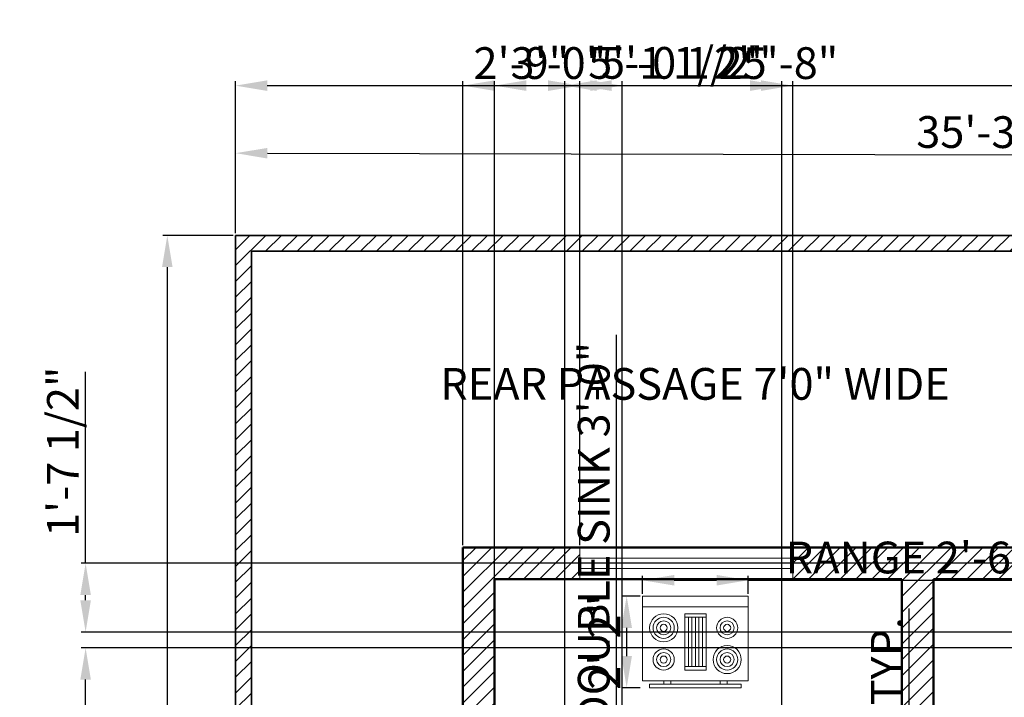
# Model space of a CAD drawing. Units: inches. Extents: x 36184 to 36805, y 18177 to 19069.
# Tile 4 of 5: x 36184 to 36463, y 18876 to 19069. Entities that reach past the tile are written whole.
import ezdxf

# ---------------------------------------------------------------- set-up
doc = ezdxf.new("R2010")
doc.units = ezdxf.units.IN
for name, color, linetype, lineweight in [('A-ANNO-DIMS', 2, 'Continuous', 18), ('A-AREA-IDEN', 7, 'Continuous', 25), ('A-EQPM', 8, 'Continuous', 18), ('A-GLAZ', 4, 'Continuous', 18), ('A-WALL', 7, 'Continuous', 50), ('C-PROP', 7, 'Continuous', 35), ('L-SITE-WALL', 7, 'Continuous', 35)]:
    doc.layers.add(name, color=color, linetype=linetype, lineweight=lineweight)
doc.layers.add('A-WALL-PATT', color=244, linetype='Continuous', lineweight=13, true_color=0x991b1e)
doc.styles.get("Standard").update_dxf_attribs({"font": 'arial.ttf'})
doc.dimstyles.new('ISO-25', dxfattribs={"dimtxt": 9, "dimasz": 9, "dimexe": 1.25, "dimexo": 0.625, "dimtad": 1, "dimdec": 1, "dimrnd": 9, "dimlunit": 3, "dimtxsty": 'Standard', "dimcen": 2.5, "dimadec": 0, "dimazin": 0, "dimtfac": 1, "dimtdec": 1, "dimtmove": 0, "dimatfit": 3, "dimfxl": 1, "dimarcsym": 0})

# ---------------------------------------------------------------- blocks, each defined once
blk = doc.blocks.new('Range-Oven - 30 in top')
for p, q in [((0, -3), (30, -3)), ((12, -6), (18, -6)), ((13, -20), (13, -6)), ((14, -6), (14, -20)), ((15, -20), (15, -6)), ((16, -6), (16, -20)), ((17, -20), (17, -6)), ((18, -20), (12, -20)), ((6, -24), (6, -25)), ((8, -25), (8, -24)), ((22, -25), (22, -24)), ((24, -24), (24, -25))]:
    blk.add_line(p, q)
for points in [[(0, -24), (0, 0), (30, 0), (30, -24)], [(12, -21), (12, -5), (18, -5), (18, -21)], [(2, -26), (2, -25), (28, -25), (28, -26)]]:
    blk.add_lwpolyline(points, close=True)
for centre, radius in [((6, -9), 4), ((6, -9), 3), ((6, -9), 2), ((6, -9), 1), ((24, -9), 3), ((24, -9), 2), ((24, -9), 1), ((6, -18), 3), ((6, -18), 2), ((24, -18), 4), ((24, -18), 3), ((24, -18), 2), ((6, -18), 1), ((24, -18), 1)]:
    blk.add_circle(centre, radius)
blk = doc.blocks.new('*D13')
at = {"layer": 'A-ANNO-DIMS', "color": 0, "lineweight": -2, "transparency": 16777216}
for p, q in [((36245.31, 19007.93), (36245.36, 19031.89)), ((36665.31, 19007.11), (36665.36, 19031.07)), ((36254.36, 19030.62), (36656.36, 19029.84))]:
    blk.add_line(p, q, dxfattribs=at)
at = {"layer": 'A-ANNO-DIMS', "color": 0, "transparency": 16777216}
for points in [[(36254.36, 19032.12), (36254.35, 19029.12), (36245.36, 19030.64)], [(36656.36, 19031.34), (36656.35, 19028.34), (36665.36, 19029.82)]]:
    blk.add_solid(points, dxfattribs=at)
at = {"layer": 'Defpoints', "color": 0, "transparency": 16777216}
for p in [(36665.36, 19029.82), (36245.31, 19007.3), (36665.31, 19006.48)]:
    blk.add_point(p, dxfattribs=at)
at = {"layer": 'A-ANNO-DIMS', "color": 0, "transparency": 16777216, "insert": (36455.37, 19035.45), "char_height": 9, "attachment_point": 5, "rotation": 359.8885}
blk.add_mtext('35\'-3"', dxfattribs=at)
blk = doc.blocks.new('*D14')
at = {"layer": 'A-ANNO-DIMS', "color": 0, "lineweight": -2, "transparency": 16777216}
for p, q in [((36244.69, 19007.3), (36224.73, 19007.3)), ((36225.98, 18998.3), (36225.98, 18420.79)), ((36244.69, 18411.79), (36224.73, 18411.79))]:
    blk.add_line(p, q, dxfattribs=at)
at = {"layer": 'A-ANNO-DIMS', "color": 0, "transparency": 16777216}
for points in [[(36224.48, 18998.3), (36227.48, 18998.3), (36225.98, 19007.3)], [(36224.48, 18420.79), (36227.48, 18420.79), (36225.98, 18411.79)]]:
    blk.add_solid(points, dxfattribs=at)
at = {"layer": 'Defpoints', "color": 0, "transparency": 16777216}
for p in [(36245.31, 19007.3), (36225.98, 18411.79), (36245.31, 18411.79)]:
    blk.add_point(p, dxfattribs=at)
at = {"layer": 'A-ANNO-DIMS', "color": 0, "transparency": 16777216, "insert": (36220.76, 18709.54), "char_height": 9, "attachment_point": 5, "rotation": 90}
blk.add_mtext('49\'-6"', dxfattribs=at)
blk = doc.blocks.new('*D28')
at = {"layer": 'A-ANNO-DIMS', "color": 0, "lineweight": -2, "transparency": 16777216}
for p, q in [((36436.4, 18801.8), (36436.4, 18901.45)), ((36431.63, 18801.8), (36437.65, 18801.8)), ((36436.4, 18774.8), (36436.4, 18792.8)), ((36431.63, 18765.8), (36437.65, 18765.8))]:
    blk.add_line(p, q, dxfattribs=at)
at = {"layer": 'A-ANNO-DIMS', "color": 0, "transparency": 16777216}
for points in [[(36434.9, 18792.8), (36437.9, 18792.8), (36436.4, 18801.8)], [(36434.9, 18774.8), (36437.9, 18774.8), (36436.4, 18765.8)]]:
    blk.add_solid(points, dxfattribs=at)
at = {"layer": 'Defpoints', "color": 0, "transparency": 16777216}
for p in [(36431, 18801.8), (36436.4, 18801.8), (36431, 18765.8)]:
    blk.add_point(p, dxfattribs=at)
at = {"layer": 'A-ANNO-DIMS', "color": 0, "transparency": 16777216, "insert": (36431.18, 18856.13), "char_height": 9, "attachment_point": 5, "rotation": 90}
blk.add_mtext('LEAF 3\'-0" TYP.', dxfattribs=at)
blk = doc.blocks.new('*D40')
at = {"layer": 'A-ANNO-DIMS', "color": 0, "lineweight": -2, "transparency": 16777216}
for p, q in [((36360.76, 18905.62), (36360.76, 18910.74)), ((36369.76, 18909.49), (36381.76, 18909.49)), ((36390.76, 18905.62), (36390.76, 18910.74)), ((36390.76, 18909.49), (36472.67, 18909.49))]:
    blk.add_line(p, q, dxfattribs=at)
at = {"layer": 'A-ANNO-DIMS', "color": 0, "transparency": 16777216}
for points in [[(36369.76, 18910.99), (36369.76, 18907.99), (36360.76, 18909.49)], [(36381.76, 18910.99), (36381.76, 18907.99), (36390.76, 18909.49)]]:
    blk.add_solid(points, dxfattribs=at)
at = {"layer": 'Defpoints', "color": 0, "transparency": 16777216}
for p in [(36390.76, 18909.49), (36360.76, 18904.99), (36390.76, 18904.99)]:
    blk.add_point(p, dxfattribs=at)
at = {"layer": 'A-ANNO-DIMS', "color": 0, "transparency": 16777216, "insert": (36436.22, 18914.77), "char_height": 9, "attachment_point": 5}
blk.add_mtext('RANGE 2\'-6"', dxfattribs=at)
blk = doc.blocks.new('*D41')
at = {"layer": 'A-ANNO-DIMS', "color": 0, "lineweight": -2, "transparency": 16777216}
for p, q in [((36360.13, 18904.99), (36355.01, 18904.99)), ((36356.26, 18887.99), (36356.26, 18895.99)), ((36360.13, 18878.99), (36355.01, 18878.99))]:
    blk.add_line(p, q, dxfattribs=at)
at = {"layer": 'A-ANNO-DIMS', "color": 0, "transparency": 16777216}
for points in [[(36354.76, 18895.99), (36357.76, 18895.99), (36356.26, 18904.99)], [(36354.76, 18887.99), (36357.76, 18887.99), (36356.26, 18878.99)]]:
    blk.add_solid(points, dxfattribs=at)
at = {"layer": 'Defpoints', "color": 0, "transparency": 16777216}
for p in [(36356.26, 18904.99), (36360.76, 18904.99), (36360.76, 18878.99)]:
    blk.add_point(p, dxfattribs=at)
at = {"layer": 'A-ANNO-DIMS', "color": 0, "transparency": 16777216, "insert": (36351.12, 18891.99), "char_height": 9, "attachment_point": 5, "rotation": 90}
blk.add_mtext('2\'-2"', dxfattribs=at)
blk = doc.blocks.new('*D42')
at = {"layer": 'A-ANNO-DIMS', "color": 0, "lineweight": -2, "transparency": 16777216}
for p, q in [((36353.36, 18857.38), (36353.36, 18979.14)), ((36348.59, 18857.38), (36354.61, 18857.38)), ((36353.36, 18830.38), (36353.36, 18848.38)), ((36348.59, 18821.38), (36354.61, 18821.38))]:
    blk.add_line(p, q, dxfattribs=at)
at = {"layer": 'A-ANNO-DIMS', "color": 0, "transparency": 16777216}
for points in [[(36351.86, 18848.38), (36354.86, 18848.38), (36353.36, 18857.38)], [(36351.86, 18830.38), (36354.86, 18830.38), (36353.36, 18821.38)]]:
    blk.add_solid(points, dxfattribs=at)
at = {"layer": 'Defpoints', "color": 0, "transparency": 16777216}
for p in [(36347.96, 18857.38), (36353.36, 18857.38), (36347.96, 18821.38)]:
    blk.add_point(p, dxfattribs=at)
at = {"layer": 'A-ANNO-DIMS', "color": 0, "transparency": 16777216, "insert": (36348.08, 18922.76), "char_height": 9, "attachment_point": 5, "rotation": 90}
blk.add_mtext('DOUBLE SINK 3\'-0"', dxfattribs=at)
blk = doc.blocks.new('*D45')
at = {"layer": 'A-ANNO-DIMS', "color": 0, "lineweight": -2, "transparency": 16777216}
for p, q in [((36245.31, 19007.93), (36245.31, 19051.05)), ((36553.31, 19007.93), (36553.31, 19051.05)), ((36254.31, 19049.8), (36544.31, 19049.8))]:
    blk.add_line(p, q, dxfattribs=at)
at = {"layer": 'A-ANNO-DIMS', "color": 0, "transparency": 16777216}
for points in [[(36254.31, 19051.3), (36254.31, 19048.3), (36245.31, 19049.8)], [(36544.31, 19051.3), (36544.31, 19048.3), (36553.31, 19049.8)]]:
    blk.add_solid(points, dxfattribs=at)
at = {"layer": 'Defpoints', "color": 0, "transparency": 16777216}
for p in [(36553.31, 19049.8), (36245.31, 19007.3), (36553.31, 19007.3)]:
    blk.add_point(p, dxfattribs=at)
at = {"layer": 'A-ANNO-DIMS', "color": 0, "transparency": 16777216, "insert": (36399.31, 19055.02), "char_height": 9, "attachment_point": 5}
blk.add_mtext('25\'-8"', dxfattribs=at)
blk = doc.blocks.new('*D49')
at = {"layer": 'A-ANNO-DIMS', "color": 0, "lineweight": -2, "transparency": 16777216}
for p, q in [((36600.19, 18890.3), (36201.56, 18890.3)), ((36202.81, 18839.3), (36202.81, 18881.3)), ((36600.19, 18830.3), (36201.56, 18830.3))]:
    blk.add_line(p, q, dxfattribs=at)
at = {"layer": 'A-ANNO-DIMS', "color": 0, "transparency": 16777216}
for points in [[(36201.31, 18881.3), (36204.31, 18881.3), (36202.81, 18890.3)], [(36201.31, 18839.3), (36204.31, 18839.3), (36202.81, 18830.3)]]:
    blk.add_solid(points, dxfattribs=at)
at = {"layer": 'Defpoints', "color": 0, "transparency": 16777216}
for p in [(36202.81, 18890.3), (36600.81, 18890.3), (36600.81, 18830.3)]:
    blk.add_point(p, dxfattribs=at)
at = {"layer": 'A-ANNO-DIMS', "color": 0, "transparency": 16777216, "insert": (36197.59, 18860.3), "char_height": 9, "attachment_point": 5, "rotation": 90}
blk.add_mtext('5\'-0"', dxfattribs=at)
blk = doc.blocks.new('*D50')
at = {"layer": 'A-ANNO-DIMS', "color": 0, "lineweight": -2, "transparency": 16777216}
for p, q in [((36202.81, 18914.3), (36202.81, 18968.6)), ((36600.19, 18914.3), (36201.56, 18914.3)), ((36202.81, 18903.8), (36202.81, 18905.3)), ((36600.19, 18894.8), (36201.56, 18894.8))]:
    blk.add_line(p, q, dxfattribs=at)
at = {"layer": 'A-ANNO-DIMS', "color": 0, "transparency": 16777216}
for points in [[(36201.31, 18905.3), (36204.31, 18905.3), (36202.81, 18914.3)], [(36201.31, 18903.8), (36204.31, 18903.8), (36202.81, 18894.8)]]:
    blk.add_solid(points, dxfattribs=at)
at = {"layer": 'Defpoints', "color": 0, "transparency": 16777216}
for p in [(36202.81, 18914.3), (36600.81, 18914.3), (36600.81, 18894.8)]:
    blk.add_point(p, dxfattribs=at)
at = {"layer": 'A-ANNO-DIMS', "color": 0, "transparency": 16777216, "insert": (36197.53, 18945.95), "char_height": 9, "attachment_point": 5, "rotation": 90}
blk.add_mtext('1\'-7 1/2"', dxfattribs=at)
blk = doc.blocks.new('*D53')
at = {"layer": 'A-ANNO-DIMS', "color": 0, "lineweight": -2, "transparency": 16777216}
for p, q in [((36342.97, 18919.43), (36342.97, 19051.05)), ((36403.35, 18919.43), (36403.35, 19051.05)), ((36351.97, 19049.8), (36394.35, 19049.8))]:
    blk.add_line(p, q, dxfattribs=at)
at = {"layer": 'A-ANNO-DIMS', "color": 0, "transparency": 16777216}
for points in [[(36351.97, 19051.3), (36351.97, 19048.3), (36342.97, 19049.8)], [(36394.35, 19051.3), (36394.35, 19048.3), (36403.35, 19049.8)]]:
    blk.add_solid(points, dxfattribs=at)
at = {"layer": 'Defpoints', "color": 0, "transparency": 16777216}
for p in [(36403.35, 19049.8), (36342.97, 18918.8), (36403.35, 18918.8)]:
    blk.add_point(p, dxfattribs=at)
at = {"layer": 'A-ANNO-DIMS', "color": 0, "transparency": 16777216, "insert": (36373.16, 19055.08), "char_height": 9, "attachment_point": 5}
blk.add_mtext('5\'-0 1/2"', dxfattribs=at)
blk = doc.blocks.new('*D54')
at = {"layer": 'A-ANNO-DIMS', "color": 0, "lineweight": -2, "transparency": 16777216}
for p, q in [((36309.81, 18919.43), (36309.81, 19051.05)), ((36342.97, 18919.43), (36342.97, 19051.05)), ((36318.81, 19049.8), (36333.97, 19049.8))]:
    blk.add_line(p, q, dxfattribs=at)
at = {"layer": 'A-ANNO-DIMS', "color": 0, "transparency": 16777216}
for points in [[(36318.81, 19051.3), (36318.81, 19048.3), (36309.81, 19049.8)], [(36333.97, 19051.3), (36333.97, 19048.3), (36342.97, 19049.8)]]:
    blk.add_solid(points, dxfattribs=at)
at = {"layer": 'Defpoints', "color": 0, "transparency": 16777216}
for p in [(36342.97, 19049.8), (36309.81, 18918.8), (36342.97, 18918.8)]:
    blk.add_point(p, dxfattribs=at)
at = {"layer": 'A-ANNO-DIMS', "color": 0, "transparency": 16777216, "insert": (36326.39, 19055.02), "char_height": 9, "attachment_point": 5}
blk.add_mtext('2\'-9"', dxfattribs=at)
blk = doc.blocks.new('*D55')
at = {"layer": 'A-ANNO-DIMS', "color": 0, "lineweight": -2, "transparency": 16777216}
for p, q in [((36318.81, 18770.93), (36318.81, 19051.05)), ((36354.96, 18770.93), (36354.96, 19051.05)), ((36327.81, 19049.8), (36345.96, 19049.8))]:
    blk.add_line(p, q, dxfattribs=at)
at = {"layer": 'A-ANNO-DIMS', "color": 0, "transparency": 16777216}
for points in [[(36327.81, 19051.3), (36327.81, 19048.3), (36318.81, 19049.8)], [(36345.96, 19051.3), (36345.96, 19048.3), (36354.96, 19049.8)]]:
    blk.add_solid(points, dxfattribs=at)
at = {"layer": 'Defpoints', "color": 0, "transparency": 16777216}
for p in [(36354.96, 19049.8), (36318.81, 18770.3), (36354.96, 18770.3)]:
    blk.add_point(p, dxfattribs=at)
at = {"layer": 'A-ANNO-DIMS', "color": 0, "transparency": 16777216, "insert": (36336.89, 19055.03), "char_height": 9, "attachment_point": 5}
blk.add_mtext('3\'-0"', dxfattribs=at)
blk = doc.blocks.new('*D60')
at = {"layer": 'A-ANNO-DIMS', "color": 0, "lineweight": -2, "transparency": 16777216}
for p, q in [((36338.76, 18403.43), (36338.76, 19051.05)), ((36400.25, 18403.43), (36400.25, 19051.05)), ((36347.76, 19049.8), (36391.25, 19049.8))]:
    blk.add_line(p, q, dxfattribs=at)
at = {"layer": 'A-ANNO-DIMS', "color": 0, "transparency": 16777216}
for points in [[(36347.76, 19051.3), (36347.76, 19048.3), (36338.76, 19049.8)], [(36391.25, 19051.3), (36391.25, 19048.3), (36400.25, 19049.8)]]:
    blk.add_solid(points, dxfattribs=at)
at = {"layer": 'Defpoints', "color": 0, "transparency": 16777216}
for p in [(36400.25, 19049.8), (36338.76, 18402.8), (36400.25, 18402.8)]:
    blk.add_point(p, dxfattribs=at)
at = {"layer": 'A-ANNO-DIMS', "color": 0, "transparency": 16777216, "insert": (36369.51, 19055.08), "char_height": 9, "attachment_point": 5}
blk.add_mtext('5\'-1 1/2"', dxfattribs=at)

msp = doc.modelspace()

# ---------------------------------------------------------------- hatches: boundary and pattern name
at = {"layer": 'A-WALL-PATT'}
h = msp.add_hatch(dxfattribs=at)
h.set_pattern_fill('ANSI31', color=256)
h.paths.add_polyline_path([(36318.81, 18555.8), (36459.81, 18555.8), (36459.81, 18705.8), (36440.41, 18705.8), (36440.41, 18696.8), (36450.81, 18696.8), (36450.81, 18564.8), (36318.81, 18564.8), (36318.81, 18591.83), (36309.81, 18591.83), (36309.81, 18525.65), (36318.81, 18525.65)], flags=17)
h.paths.add_polyline_path([(36318.81, 18455.41), (36309.81, 18455.41), (36309.81, 18402.8), (36338.76, 18402.8), (36338.76, 18411.8), (36318.81, 18411.8)], flags=17)
h.paths.add_polyline_path([(36423.09, 18411.8), (36400.25, 18411.8), (36400.25, 18402.8), (36423.09, 18402.8)], flags=17)
h.paths.add_polyline_path([(36492.81, 18478.27), (36496.58, 18481.34), (36494.6, 18487.78), (36492.81, 18486.25), (36483.81, 18479.84), (36483.81, 18411.8), (36473.38, 18411.8), (36473.38, 18402.8), (36483.81, 18402.8), (36483.81, 18356.3), (36483.81, 18347.3), (36519.81, 18347.3), (36524.04, 18347.3), (36524.04, 18356.3), (36492.81, 18356.3)], flags=17)
h.paths.add_polyline_path([(36665.31, 18608.3), (36660.81, 18608.3), (36660.81, 18557.3), (36646.76, 18557.3), (36646.76, 18552.8), (36660.81, 18552.8), (36660.81, 18504.8), (36650.24, 18504.8), (36650.24, 18500.3), (36660.81, 18500.3), (36660.81, 18356.3), (36622.58, 18356.3), (36622.58, 18347.3), (36665.31, 18347.3)])
h.paths.add_polyline_path([(36608.31, 18509.3), (36519.81, 18509.3), (36513.55, 18503.95), (36517.84, 18498.69), (36519.81, 18500.3), (36608.31, 18500.3)])
h.paths.add_polyline_path([(36254.31, 18411.79), (36249.81, 18411.79), (36249.81, 19002.8), (36553.31, 19002.8), (36553.31, 19007.3), (36245.31, 19007.3), (36245.31, 18288.82), (36254.31, 18288.82)])
h.paths.add_polyline_path([(36342.97, 18918.8), (36309.81, 18918.8), (36309.81, 18747.12), (36314.31, 18747.12), (36314.31, 18765.8), (36384.81, 18765.8), (36384.81, 18701.3), (36350.57, 18701.3), (36350.57, 18696.8), (36396.53, 18696.8), (36396.53, 18705.8), (36389.31, 18705.8), (36389.31, 18761.3), (36393.31, 18761.3), (36393.31, 18770.3), (36384.81, 18770.3), (36318.81, 18770.3), (36318.81, 18909.8), (36342.97, 18909.8)], flags=17)
h.paths.add_polyline_path([(36469.15, 18918.8), (36403.35, 18918.8), (36403.35, 18909.8), (36434.31, 18909.8), (36434.31, 18770.3), (36431, 18770.3), (36431, 18761.3), (36449.29, 18761.3), (36449.29, 18770.3), (36443.31, 18770.3), (36443.31, 18909.8), (36469.15, 18909.8)], flags=17)
h.paths.add_polyline_path([(36557.81, 18953.44), (36553.31, 18953.44), (36553.31, 18918.8), (36527.35, 18918.8), (36527.35, 18909.8), (36553.31, 18909.8), (36562.16, 18909.8), (36562.16, 18914.3), (36557.81, 18914.3)])
h.paths.add_polyline_path([(36665.31, 19007.3), (36553.31, 19007.3), (36553.31, 19002.8), (36553.31, 18989.93), (36557.81, 18989.93), (36557.81, 19002.8), (36660.81, 19002.8), (36660.81, 18765.8), (36656.73, 18765.8), (36656.73, 18761.3), (36660.81, 18761.3), (36660.81, 18617.3), (36654.49, 18617.3), (36654.49, 18608.3), (36665.31, 18608.3)])
h.paths.add_polyline_path([(36600.81, 18890.3), (36596.31, 18890.3), (36596.31, 18770.3), (36487.63, 18770.3), (36487.63, 18761.3), (36519.81, 18761.3), (36519.81, 18756.26), (36528.81, 18756.26), (36528.81, 18761.3), (36634.81, 18761.3), (36634.81, 18765.8), (36600.81, 18765.8), (36600.81, 18825.8), (36660.81, 18825.8), (36660.81, 18830.3), (36600.81, 18830.3)])
h.paths.add_polyline_path([(36600.81, 18914.3), (36596.31, 18914.3), (36591.43, 18914.3), (36591.43, 18909.8), (36596.31, 18909.8), (36596.31, 18890.3), (36660.81, 18890.3), (36660.81, 18894.8), (36600.81, 18894.8)], flags=17)
h.paths.add_polyline_path([(36623.57, 18617.3), (36528.81, 18617.3), (36528.81, 18717.38), (36519.81, 18717.38), (36519.81, 18608.3), (36608.31, 18608.3), (36608.31, 18603.13), (36617.31, 18603.13), (36617.31, 18608.3), (36623.57, 18608.3)])
h.paths.add_polyline_path([(36602.02, 18898.95), (36663.11, 18898.95), (36663.11, 18913.37), (36602.02, 18913.37)], flags=25)

# ---------------------------------------------------------------- linework, layer by layer
at = {"layer": 'A-GLAZ'}
for p, q in [((36342.97, 18918.8), (36342.97, 18909.8)), ((36403.35, 18918.8), (36403.35, 18909.8)), ((36403.35, 18915.8), (36342.97, 18915.8)), ((36403.35, 18912.8), (36342.97, 18912.8))]:
    msp.add_line(p, q, dxfattribs=at)
at = {"layer": 'A-WALL'}
for p, q in [((36553.31, 18918.8), (36309.81, 18918.8)), ((36309.81, 18918.8), (36309.81, 18402.8)), ((36318.81, 18909.8), (36318.81, 18770.3)), ((36434.31, 18909.8), (36318.81, 18909.8)), ((36434.31, 18770.3), (36434.31, 18909.8)), ((36553.31, 18909.8), (36443.31, 18909.8)), ((36443.31, 18770.3), (36443.31, 18909.8))]:
    msp.add_line(p, q, dxfattribs=at)
at = {"layer": 'C-PROP'}
for p, q in [((36665.31, 19007.3), (36245.31, 19007.3)), ((36245.31, 19007.3), (36245.31, 18227.3))]:
    msp.add_line(p, q, dxfattribs=at)
at = {"layer": 'L-SITE-WALL'}
for p, q in [((36249.81, 19002.8), (36249.81, 18411.79)), ((36553.31, 19002.8), (36249.81, 19002.8))]:
    msp.add_line(p, q, dxfattribs=at)

# ---------------------------------------------------------------- block references
at = {"layer": 'A-EQPM'}
msp.add_blockref('Range-Oven - 30 in top', (36360.76, 18904.99), dxfattribs=at)

# ---------------------------------------------------------------- texts
at = {"layer": 'A-AREA-IDEN', "insert": (36303.39, 18969.69), "char_height": 9, "attachment_point": 1}
msp.add_mtext_dynamic_manual_height_columns('REAR PASSAGE 7\'0" WIDE', width=233.2566, gutter_width=12.5, heights=[0], dxfattribs=at)

# ---------------------------------------------------------------- dimensions: what is measured, and where the dimension line sits
at = {"layer": 'A-ANNO-DIMS'}
for base, p1, p2, picture, middle in [((36400.25, 19049.8), (36338.76, 18402.8), (36400.25, 18402.8), '*D60', (36369.51, 19055.08)), ((36403.35, 19049.8), (36342.97, 18918.8), (36403.35, 18918.8), '*D53', (36373.16, 19055.08)), ((36553.31, 19049.8), (36245.31, 19007.3), (36553.31, 19007.3), '*D45', (36399.31, 19055.02)), ((36342.97, 19049.8), (36309.81, 18918.8), (36342.97, 18918.8), '*D54', (36326.39, 19055.02)), ((36354.9601, 19049.8021), (36318.8117, 18770.3021), (36354.9601, 18770.3021), '*D55', (36336.8859, 19055.0254))]:
    dim = msp.add_linear_dim(base=base, p1=p1, p2=p2, dimstyle='ISO-25', override={"dimdec": 1, "dimlfac": 1, "dimrnd": 0, "dimzin": 1, "dimdsep": 46, "dimlunit": 4, "dimfrac": 2}, dxfattribs=at)
    dim.commit()
    dim.dimension.update_dxf_attribs({"geometry": picture, "text_midpoint": middle})
dim = msp.add_aligned_dim(p1=(36245.31, 19007.3), p2=(36665.31, 19006.48), distance=23.33, dimstyle='ISO-25', override={"dimclrd": 0, "dimclre": 0, "dimclrt": 0}, dxfattribs=at)
dim.commit()
dim.dimension.update_dxf_attribs({"geometry": '*D13', "text_midpoint": (36455.37, 19035.45)})
for base, p1, p2, override, picture, middle in [((36225.98, 18411.79), (36245.31, 19007.3), (36245.31, 18411.79), {"dimclrd": 0, "dimclre": 0, "dimclrt": 0}, '*D14', (36220.76, 18709.54)), ((36202.81, 18914.3), (36600.81, 18894.8), (36600.81, 18914.3), {"dimdec": 1, "dimlfac": 1, "dimrnd": 0, "dimzin": 1, "dimdsep": 46, "dimlunit": 4, "dimfrac": 2}, '*D50', (36197.53, 18945.95)), ((36356.26, 18904.99), (36360.76, 18878.99), (36360.76, 18904.99), {"dimdec": 1, "dimlfac": 1, "dimrnd": 0, "dimzin": 1, "dimdsep": 46, "dimlunit": 4, "dimfrac": 2}, '*D41', (36351.12, 18891.99)), ((36202.81, 18890.3), (36600.81, 18830.3), (36600.81, 18890.3), {"dimdec": 1, "dimlfac": 1, "dimrnd": 0, "dimzin": 1, "dimdsep": 46, "dimlunit": 4, "dimfrac": 2}, '*D49', (36197.59, 18860.3))]:
    dim = msp.add_linear_dim(base=base, p1=p1, p2=p2, angle=90, dimstyle='ISO-25', override=override, dxfattribs=at)
    dim.commit()
    dim.dimension.update_dxf_attribs({"geometry": picture, "text_midpoint": middle})
for base, p1, p2, text, picture, middle in [((36353.36, 18857.38), (36347.96, 18821.38), (36347.96, 18857.38), 'DOUBLE SINK <>', '*D42', (36348.08, 18922.76)), ((36436.4, 18801.8), (36431, 18765.8), (36431, 18801.8), 'LEAF <> TYP.', '*D28', (36431.18, 18856.13))]:
    dim = msp.add_linear_dim(base=base, p1=p1, p2=p2, angle=90, text=text, dimstyle='ISO-25', override={"dimdec": 1, "dimlfac": 1, "dimrnd": 0, "dimzin": 1, "dimdsep": 46, "dimlunit": 4, "dimfrac": 2}, dxfattribs=at)
    dim.commit()
    dim.dimension.update_dxf_attribs({"geometry": picture, "text_midpoint": middle})
dim = msp.add_linear_dim(base=(36390.76, 18909.49), p1=(36360.76, 18904.99), p2=(36390.76, 18904.99), text='RANGE <>', dimstyle='ISO-25', override={"dimdec": 1, "dimlfac": 1, "dimrnd": 0, "dimzin": 1, "dimdsep": 46, "dimlunit": 4, "dimfrac": 2}, dxfattribs=at)
dim.commit()
dim.dimension.update_dxf_attribs({"geometry": '*D40', "text_midpoint": (36436.22, 18914.77)})

doc.saveas('drawing.dxf')
